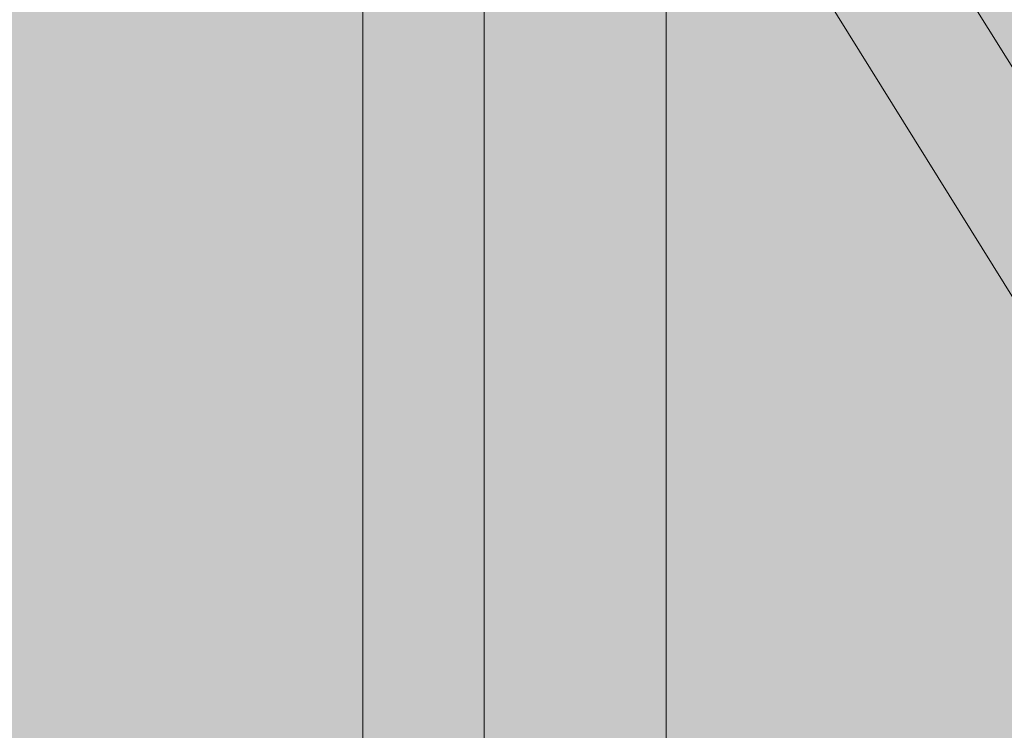
# Model space of a CAD drawing. Units: millimetres. Extents: x 11032 to 26788, y 3406 to 24505.
# Tile 45 of 78: x 15518 to 15924, y 15746 to 16039. Entities that reach past the tile are written whole.
import ezdxf

# ---------------------------------------------------------------- set-up
doc = ezdxf.new("R2010")
doc.units = ezdxf.units.MM
doc.header["$MEASUREMENT"] = 0
for name, color, linetype, lineweight in [('A-ANNO-DIMS', 2, 'Continuous', 18), ('A-GLAZ', 250, 'Continuous', 20), ('A-ROOF', 7, 'Continuous', 30), ('A-WALL', 7, 'Continuous', 35)]:
    doc.layers.add(name, color=color, linetype=linetype, lineweight=lineweight)
for name, color, linetype, lineweight, true_color in [('A-GLAZ-FRAM-PATT', 250, 'Continuous', 13, 0x262627), ('A-ROOF-PATT', 9, 'Continuous', 13, 0xc7c8ca), ('A-WALL-INTR-PATT', 251, 'Continuous', 13, 0x6c6b6a)]:
    doc.layers.add(name, color=color, linetype=linetype, lineweight=lineweight, true_color=true_color)
doc.styles.get("Standard").update_dxf_attribs({"font": 'arial.ttf'})
doc.dimstyles.get("Standard").update_dxf_attribs({"dimtxt": 150, "dimasz": 100, "dimexe": 10, "dimexo": 5, "dimgap": 5, "dimtad": 0, "dimtih": 1, "dimtoh": 1, "dimdec": 0, "dimzin": 0, "dimdsep": 46, "dimtxsty": 'Standard', "dimcen": 0.09, "dimadec": 0, "dimazin": 0, "dimtfac": 1, "dimtdec": 0, "dimtofl": 0, "dimtmove": 0, "dimatfit": 3, "dimfxl": 1, "dimtolj": 1, "dimtzin": 0, "dimarcsym": 0})

# ---------------------------------------------------------------- blocks, each defined once
blk = doc.blocks.new('*D36')
at = {"layer": 'A-ANNO-DIMS', "color": 0, "lineweight": -2, "transparency": 16777216}
for p, q in [((12301.26, 17115.89), (12301.26, 24416.86)), ((25397.4, 4466.4), (25397.4, 24416.86)), ((12401.26, 24406.86), (18569.2, 24406.86)), ((25297.4, 24406.86), (19129.47, 24406.86))]:
    blk.add_line(p, q, dxfattribs=at)
at = {"layer": 'A-ANNO-DIMS', "color": 0, "transparency": 16777216}
for points in [[(12401.26, 24423.52), (12401.26, 24390.19), (12301.26, 24406.86)], [(25297.4, 24423.52), (25297.4, 24390.19), (25397.4, 24406.86)]]:
    blk.add_solid(points, dxfattribs=at)
at = {"layer": 'Defpoints', "color": 0, "transparency": 16777216}
for p in [(25397.4, 24406.86), (12301.26, 17110.89), (25397.4, 4461.4)]:
    blk.add_point(p, dxfattribs=at)
at = {"layer": 'A-ANNO-DIMS', "color": 0, "transparency": 16777216, "insert": (18849.33, 24406.86), "char_height": 150, "attachment_point": 5}
blk.add_mtext('\\A1;13096', dxfattribs=at)
blk = doc.blocks.new('*D37')
at = {"layer": 'A-ANNO-DIMS', "color": 0, "lineweight": -2, "transparency": 16777216}
for p, q in [((18087.74, 23450.36), (11334.76, 23450.36)), ((11344.76, 23350.36), (11344.76, 14037.46)), ((11344.76, 4561.4), (11344.76, 13874.29)), ((12927.66, 4461.4), (11334.76, 4461.4))]:
    blk.add_line(p, q, dxfattribs=at)
at = {"layer": 'A-ANNO-DIMS', "color": 0, "transparency": 16777216}
for points in [[(11328.1, 23350.36), (11361.43, 23350.36), (11344.76, 23450.36)], [(11328.1, 4561.4), (11361.43, 4561.4), (11344.76, 4461.4)]]:
    blk.add_solid(points, dxfattribs=at)
at = {"layer": 'Defpoints', "color": 0, "transparency": 16777216}
for p in [(11344.76, 23450.36), (18092.74, 23450.36), (12932.66, 4461.4)]:
    blk.add_point(p, dxfattribs=at)
at = {"layer": 'A-ANNO-DIMS', "color": 0, "transparency": 16777216, "insert": (11344.76, 13955.88), "char_height": 150, "attachment_point": 5}
blk.add_mtext('\\A1;18989', dxfattribs=at)
blk = doc.blocks.new('*D57')
at = {"layer": 'A-ANNO-DIMS', "color": 0, "lineweight": -2, "transparency": 16777216}
for p, q in [((14994.7, 7266.4), (14994.7, 24416.86)), ((20894.7, 7266.4), (20894.7, 24416.86)), ((15094.7, 24406.86), (17715.98, 24406.86)), ((20794.7, 24406.86), (18173.42, 24406.86))]:
    blk.add_line(p, q, dxfattribs=at)
at = {"layer": 'A-ANNO-DIMS', "color": 0, "transparency": 16777216}
for points in [[(15094.7, 24423.52), (15094.7, 24390.19), (14994.7, 24406.86)], [(20794.7, 24423.52), (20794.7, 24390.19), (20894.7, 24406.86)]]:
    blk.add_solid(points, dxfattribs=at)
at = {"layer": 'Defpoints', "color": 0, "transparency": 16777216}
for p in [(20894.7, 24406.86), (14994.7, 7261.4), (20894.7, 7261.4)]:
    blk.add_point(p, dxfattribs=at)
at = {"layer": 'A-ANNO-DIMS', "color": 0, "transparency": 16777216, "insert": (17944.7, 24406.86), "char_height": 150, "attachment_point": 5}
blk.add_mtext('\\A1;5900', dxfattribs=at)
blk = doc.blocks.new('*D60')
at = {"layer": 'A-ANNO-DIMS', "color": 0, "lineweight": -2, "transparency": 16777216}
for p, q in [((14994.7, 7266.4), (14994.7, 24416.86)), ((16344.7, 7266.4), (16344.7, 24416.86)), ((15094.7, 24406.86), (15448.04, 24406.86)), ((16244.7, 24406.86), (15891.36, 24406.86))]:
    blk.add_line(p, q, dxfattribs=at)
at = {"layer": 'A-ANNO-DIMS', "color": 0, "transparency": 16777216}
for points in [[(15094.7, 24423.52), (15094.7, 24390.19), (14994.7, 24406.86)], [(16244.7, 24423.52), (16244.7, 24390.19), (16344.7, 24406.86)]]:
    blk.add_solid(points, dxfattribs=at)
at = {"layer": 'Defpoints', "color": 0, "transparency": 16777216}
for p in [(16344.7, 24406.86), (14994.7, 7261.4), (16344.7, 7261.4)]:
    blk.add_point(p, dxfattribs=at)
at = {"layer": 'A-ANNO-DIMS', "color": 0, "transparency": 16777216, "insert": (15669.7, 24406.86), "char_height": 150, "attachment_point": 5}
blk.add_mtext('\\A1;1350', dxfattribs=at)

msp = doc.modelspace()

# ---------------------------------------------------------------- hatches: boundary and pattern name
at = {"layer": 'A-GLAZ-FRAM-PATT'}
h = msp.add_hatch(color=256, dxfattribs=at)
edge = h.paths.add_edge_path()
edge.add_line((15284.393, 17051.32), (15084.393, 17001.32))
edge.add_line((15084.393, 17001.32), (15084.393, 15951.32))
edge.add_spline(control_points=[(15084.393, 15951.32), (15157.266, 15924.219), (15224.458, 15897.808), (15284.393, 15870.289)], knot_values=[511.9490104, 511.9490104, 511.9490104, 511.9490104, 697.3715979, 697.3715979, 697.3715979, 697.3715979], degree=3, periodic=0)
edge.add_line((15284.393, 15870.289), (15284.393, 17051.32))
edge = h.paths.add_edge_path()
edge.add_line((15659.393, 16354.387), (15459.393, 16675.629))
edge.add_line((15459.393, 16675.629), (15459.393, 15771.505))
edge.add_spline(control_points=[(15459.393, 15771.505), (15501.891, 15741.568), (15571.096, 15682.692), (15632.72, 15612.509), (15659.393, 15578.299)], knot_values=[905.064582, 905.064582, 905.064582, 905.064582, 1079.4682707, 1223.1584353, 1223.1584353, 1223.1584353, 1223.1584353], degree=3, periodic=0)
edge.add_line((15659.393, 15578.299), (15659.393, 16354.387))
h.paths.add_polyline_path([(15284.393, 17051.32), (15284.393, 16956.717), (15784.393, 16153.61), (15784.393, 16248.213)])
h = msp.add_hatch(color=256, dxfattribs=at)
edge = h.paths.add_edge_path()
edge.add_spline(control_points=[(15409.393, 16728.446), (15384.197, 16718.122), (15359.177, 16707.259), (15334.393, 16695.842)], knot_values=[2052.6714029, 2052.6714029, 2052.6714029, 2052.6714029, 2131.0201637, 2131.0201637, 2131.0201637, 2131.0201637], degree=3, periodic=0)
edge.add_line((15334.393, 16695.842), (15334.393, 15846.165))
edge.add_spline(control_points=[(15334.393, 15846.165), (15360.99, 15832.635), (15385.89, 15818.741), (15409.393, 15804.345)], knot_values=[750.8383504, 750.8383504, 750.8383504, 750.8383504, 839.4758736, 839.4758736, 839.4758736, 839.4758736], degree=3, periodic=0)
edge.add_line((15409.393, 15804.345), (15409.393, 16728.446))
edge = h.paths.add_edge_path()
edge.add_line((15784.393, 16153.61), (15709.393, 16274.076))
edge.add_line((15709.393, 16274.076), (15709.393, 15509.31))
edge.add_spline(control_points=[(15709.393, 15509.31), (15712.398, 15504.862), (15738.373, 15465.922), (15763.422, 15424.165), (15784.393, 15385.996)], knot_values=[1315.3424293, 1315.3424293, 1315.3424293, 1315.3424293, 1332.3824154, 1463.2850479, 1463.2850479, 1463.2850479, 1463.2850479], degree=3, periodic=0)
edge.add_line((15784.393, 15385.996), (15784.393, 16153.61))
h = msp.add_hatch(color=256, dxfattribs=at)
edge = h.paths.add_edge_path()
edge.add_line((15784.393, 16248.213), (15784.393, 16153.61))
edge.add_line((15784.393, 16153.61), (16560.042, 14907.752))
edge.add_spline(control_points=[(16560.042, 14907.752), (16569.192, 14907.664), (16578.343, 14907.575), (16587.493, 14907.486), (16598.103, 14907.383), (16608.713, 14907.281), (16619.296, 14907.181)], knot_values=[1012.2878735, 1012.2878735, 1012.2878735, 1012.2878735, 1027.155312, 1027.155312, 1027.155312, 1044.3939449, 1044.3939449, 1044.3939449, 1044.3939449], degree=3, periodic=0)
edge.add_line((16619.296, 14907.181), (15784.393, 16248.213))
at = {"layer": 'A-ROOF-PATT'}
h = msp.add_hatch(color=256, dxfattribs=at)
edge = h.paths.add_edge_path()
edge.add_spline(control_points=[(17532.827, 17324.837), (17391.335, 17349.016), (16840.872, 17494.912), (16080.055, 18069.544), (14738.803, 18299.641), (13382.429, 18838.336), (12580.532, 17870.207), (12430.422, 17563.822)], knot_values=[2977.6027945, 2977.6027945, 2977.6027945, 2977.6027945, 3438.1840601, 4811.6463022, 5622.8675483, 7588.0288188, 8560.6685791, 8560.6685791, 8560.6685791, 8560.6685791], degree=3, periodic=0)
edge.add_spline(control_points=[(12430.422, 17563.822), (12437.904, 17573.36), (12445.386, 17582.899), (12452.869, 17592.437), (12452.869, 17592.438), (12452.869, 17592.438), (12452.869, 17592.438)], knot_values=[1408.564138, 1408.564138, 1408.564138, 1408.564138, 1444.85989, 1444.85989, 1444.85989, 1444.8601183, 1444.8601183, 1444.8601183, 1444.8601183], degree=3, periodic=0)
edge.add_spline(control_points=[(12452.869, 17592.438), (12555.432, 17723.185), (12736.557, 17929.686), (13044.86, 18114.643), (13219.943, 18189.644), (13299.92, 18220.646)], knot_values=[339.318246, 339.318246, 339.318246, 339.318246, 836.8349967, 1151.2512933, 1408.564138, 1408.564138, 1408.564138, 1408.564138], degree=3, periodic=0)
edge.add_spline(control_points=[(13299.92, 18220.646), (13299.998, 18220.689), (13300.077, 18220.732), (13319.738, 18231.488), (13339.24, 18241.402), (13388.645, 18264.703), (13418.466, 18277.069), (13478.019, 18298.648), (13507.751, 18307.861), (13544.561, 18317.488), (13551.584, 18319.245), (13558.612, 18320.924)], knot_values=[3783.8950972, 3783.8950972, 3783.8950972, 3783.8950972, 3784.1737101, 3784.1737101, 3853.4666747, 3853.4666747, 3960.2401917, 3960.2401917, 4067.0137087, 4067.0137087, 4092.1744649, 4092.1744649, 4092.1744649, 4092.1744649], degree=3, periodic=0)
edge.add_spline(control_points=[(13558.612, 18320.924), (13581.407, 18326.373), (13604.25, 18331.007), (13657.184, 18339.957), (13687.338, 18343.732), (13748.098, 18348.892), (13778.704, 18350.276), (13840.46, 18350.833), (13871.609, 18350.005), (13934.496, 18346.313), (13966.232, 18343.449), (14030.297, 18335.871), (14062.625, 18331.158), (14127.853, 18320.088), (14160.753, 18313.73), (14241.357, 18296.556), (14289.343, 18284.997), (14386.31, 18259.688), (14435.291, 18245.941), (14534.161, 18217.034), (14584.049, 18201.875), (14684.682, 18170.964), (14735.427, 18155.212), (14837.763, 18123.971), (14889.354, 18108.482), (14954.971, 18089.677), (14968.586, 18085.823), (14992.391, 18079.184), (15002.566, 18076.376), (15021.739, 18071.153), (15030.731, 18068.729), (15047.707, 18064.21), (15055.694, 18062.106), (15079.815, 18055.825), (15095.905, 18051.728), (15143.966, 18039.717), (15175.729, 18032.084), (15254.84, 18013.501), (15301.798, 18002.866), (15394.186, 17981.845), (15439.615, 17971.459), (15528.833, 17950.135), (15572.62, 17939.197), (15658.477, 17916.021), (15700.546, 17903.785), (15753.633, 17886.734), (15765.446, 17882.835), (15786.574, 17875.653), (15795.915, 17872.404), (15810.108, 17867.349), (15814.99, 17865.588), (15824.736, 17862.029), (15829.611, 17860.226), (15844.241, 17854.75), (15854.002, 17851.008), (15883.312, 17839.521), (15902.885, 17831.512), (15966.355, 17804.548), (16010.39, 17784.302), (16098.838, 17741.267), (16143.25, 17718.478), (16232.497, 17671.098), (16277.332, 17646.507), (16367.515, 17596.295), (16412.862, 17570.676), (16504.202, 17519.209), (16550.194, 17493.362), (16643.009, 17442.263), (16689.831, 17417.011), (16756.517, 17382.472), (16775.937, 17372.58), (16795.455, 17362.84)], knot_values=[4092.1744649, 4092.1744649, 4092.1744649, 4092.1744649, 4173.7872258, 4173.7872258, 4280.5607428, 4280.5607428, 4387.3342598, 4387.3342598, 4494.1077768, 4494.1077768, 4600.8812939, 4600.8812939, 4707.6548109, 4707.6548109, 4814.4283279, 4814.4283279, 4967.1262405, 4967.1262405, 5119.8241531, 5119.8241531, 5272.5220657, 5272.5220657, 5425.2199783, 5425.2199783, 5577.9178908, 5577.9178908, 5617.7853319, 5617.7853319, 5647.4648479, 5647.4648479, 5673.611025, 5673.611025, 5696.747607, 5696.747607, 5743.6818903, 5743.6818903, 5837.5504571, 5837.5504571, 5979.7261046, 5979.7261046, 6121.9017521, 6121.9017521, 6264.0773996, 6264.0773996, 6406.2530471, 6406.2530471, 6447.2585849, 6447.2585849, 6480.0420882, 6480.0420882, 6497.3077062, 6497.3077062, 6514.5733242, 6514.5733242, 6549.1045602, 6549.1045602, 6618.1670322, 6618.1670322, 6772.6610171, 6772.6610171, 6927.155002, 6927.155002, 7081.6489869, 7081.6489869, 7236.1429718, 7236.1429718, 7390.6369567, 7390.6369567, 7545.1309416, 7545.1309416, 7608.1992868, 7608.1992868, 7608.1992868, 7608.1992868], degree=3, periodic=0)
edge.add_spline(control_points=[(16795.455, 17362.84), (16814.335, 17349.456), (16832.897, 17336.263), (16873.225, 17307.197), (16894.778, 17291.386), (16936.221, 17259.941), (16956.11, 17244.308), (16993.863, 17213.094), (17011.726, 17197.514), (17041.993, 17169.265), (17054.791, 17156.601), (17078.762, 17131.225), (17089.933, 17118.516), (17110.618, 17092.991), (17120.131, 17080.178), (17130.17, 17065.264), (17131.487, 17063.277), (17133.77, 17059.776), (17134.746, 17058.261), (17136.69, 17055.205), (17137.657, 17053.668), (17140.539, 17049.025), (17142.438, 17045.89), (17148.068, 17036.367), (17151.732, 17029.859), (17163.03, 17008.788), (17170.335, 16993.646), (17184.087, 16961.978), (17190.534, 16945.453), (17202.562, 16911.165), (17208.142, 16893.402), (17218.448, 16856.821), (17223.173, 16838.003), (17231.801, 16799.51), (17235.705, 16779.837), (17241.533, 16746.739), (17243.676, 16733.5), (17247.718, 16706.37), (17249.608, 16692.472), (17252.066, 16672.69), (17252.761, 16666.875), (17254.1, 16655.226), (17254.744, 16649.4), (17256.596, 16631.917), (17257.727, 16620.254), (17260.823, 16585.238), (17262.489, 16561.858), (17266.551, 16488.654), (17267.658, 16438.661), (17267.349, 16375.228), (17267.193, 16362.07), (17266.95, 16348.891)], knot_values=[15.1130472, 15.1130472, 15.1130472, 15.1130472, 82.6995146, 82.6995146, 165.3990291, 165.3990291, 248.0985437, 248.0985437, 330.7980583, 330.7980583, 397.9419458, 397.9419458, 465.0858333, 465.0858333, 532.2297209, 532.2297209, 542.533741, 542.533741, 550.3568158, 550.3568158, 558.1798906, 558.1798906, 573.8260402, 573.8260402, 605.1183395, 605.1183395, 672.7640614, 672.7640614, 740.4097834, 740.4097834, 808.0555054, 808.0555054, 875.7012273, 875.7012273, 943.3469493, 943.3469493, 987.6613492, 987.6613492, 1033.4121612, 1033.4121612, 1052.3850876, 1052.3850876, 1071.358014, 1071.358014, 1109.3038668, 1109.3038668, 1185.1955724, 1185.1955724, 1346.4419026, 1346.4419026, 1388.5586631, 1388.5586631, 1388.5586631, 1388.5586631], degree=3, periodic=0)
edge.add_spline(control_points=[(17266.95, 16348.891), (17266.95, 16348.891), (17266.95, 16348.891), (17266.95, 16348.891), (17253.182, 15602.417), (17239.414, 14855.943), (17225.646, 14109.469)], knot_values=[1388.5586631, 1388.5586631, 1388.5586631, 1388.5586631, 1388.5589654, 1388.5589654, 1388.5589654, 3774.0767661, 3774.0767661, 3774.0767661, 3774.0767661], degree=3, periodic=0)
edge.add_spline(control_points=[(17225.646, 14109.469), (17226.198, 14109.827), (17226.748, 14110.185), (17242.065, 14120.191), (17255.956, 14130.116), (17274.422, 14144.286), (17279.609, 14148.386), (17284.686, 14152.511)], knot_values=[1926.3423968, 1926.3423968, 1926.3423968, 1926.3423968, 1927.316729, 1927.316729, 1953.5121761, 1953.5121761, 1964.0732348, 1964.0732348, 1964.0732348, 1964.0732348], degree=3, periodic=0)
edge.add_spline(control_points=[(17284.686, 14152.511), (17315.791, 14194.761), (17384.413, 14446.273), (17407.128, 14793.401), (17407.093, 15295.84), (17423.274, 15626.362), (17415.601, 15782.507)], knot_values=[0, 0, 0, 0, 163.2554674, 619.2296767, 1171.8624483, 1621.6355562, 1621.6355562, 1621.6355562, 1621.6355562], degree=3, periodic=0)
edge.add_spline(control_points=[(17415.601, 15782.507), (17438.21, 16077.57), (17410.495, 16533.484), (17390.893, 17030.649), (17301.082, 17169.349)], knot_values=[543.9784753, 543.9784753, 543.9784753, 543.9784753, 1452.9852767, 1960.0114926, 1960.0114926, 1960.0114926, 1960.0114926], degree=3, periodic=0)
edge.add_spline(control_points=[(17301.082, 17169.349), (17346.58, 17157.64), (17392.235, 17147.336), (17467.161, 17132.609), (17496.336, 17127.412), (17525.58, 17122.709)], knot_values=[8131.593939, 8131.593939, 8131.593939, 8131.593939, 8269.7349273, 8269.7349273, 8357.5016646, 8357.5016646, 8357.5016646, 8357.5016646], degree=3, periodic=0)
edge.add_line((17525.58, 17122.709), (17532.827, 17324.837))
edge = h.paths.add_edge_path(flags=17)
edge.add_spline(control_points=[(13340.537, 14602.706), (13316.172, 14726.456), (13323.666, 14932.342), (13637.836, 15081.117), (13863.248, 15171.051), (14002.1, 15224.503), (14058.539, 15244.876)], knot_values=[680.8931862, 680.8931862, 680.8931862, 680.8931862, 1033.4728289, 1337.4008326, 1604.7214264, 1784.2944722, 1784.2944722, 1784.2944722, 1784.2944722], degree=3, periodic=0)
edge.add_spline(control_points=[(14058.539, 15244.876), (14058.289, 15275.236), (14057.634, 15305.434), (14055.312, 15376.527), (14053.359, 15417.248), (14048.642, 15497.048), (14045.89, 15536.143), (14042.888, 15574.619)], knot_values=[6573.1065419, 6573.1065419, 6573.1065419, 6573.1065419, 6636.7330012, 6636.7330012, 6723.8890547, 6723.8890547, 6809.6328771, 6809.6328771, 6809.6328771, 6809.6328771], degree=3, periodic=0)
edge.add_spline(control_points=[(14042.888, 15574.619), (13546.54, 15403.221), (13074.735, 15143.241), (13277.36, 14695.339), (13340.537, 14602.706)], knot_values=[503.7925783, 503.7925783, 503.7925783, 503.7925783, 1728.1787606, 2051.34844, 2051.34844, 2051.34844, 2051.34844], degree=3, periodic=0)
h = msp.add_hatch(color=256, dxfattribs=at)
h.set_gradient(color1=(254, 234, 185), color2=(254, 204, 102), name='HEMISPHERICAL')
edge = h.paths.add_edge_path()
edge.add_line((15084.393, 17001.32), (15284.393, 17051.32))
edge.add_line((15284.393, 17051.32), (15470.537, 16752.334))
edge.add_spline(control_points=[(15470.537, 16752.334), (15683.311, 16831.508), (16106.827, 16912.335), (16625.609, 16876.997), (17083.498, 16357.78), (17257.801, 16180.113)], knot_values=[0, 0, 0, 0, 655.2936334, 1252.0157838, 1989.6162859, 1989.6162859, 1989.6162859, 1989.6162859], degree=3, periodic=0)
edge.add_spline(control_points=[(17257.801, 16180.113), (17260.851, 16236.372), (17263.9, 16292.632), (17266.95, 16348.891)], knot_values=[1132.9967717, 1132.9967717, 1132.9967717, 1132.9967717, 1198.0464225, 1198.0464225, 1198.0464225, 1198.0464225], degree=3, periodic=0)
edge.add_spline(control_points=[(17266.95, 16348.891), (17267.193, 16362.07), (17267.349, 16375.228), (17267.658, 16438.661), (17266.551, 16488.654), (17262.489, 16561.858), (17260.823, 16585.238), (17257.727, 16620.254), (17256.596, 16631.917), (17254.744, 16649.4), (17254.1, 16655.226), (17252.761, 16666.875), (17252.066, 16672.69), (17249.608, 16692.472), (17247.718, 16706.37), (17243.676, 16733.5), (17241.533, 16746.739), (17235.705, 16779.837), (17231.801, 16799.51), (17223.173, 16838.003), (17218.448, 16856.821), (17208.142, 16893.402), (17202.562, 16911.165), (17190.534, 16945.453), (17184.087, 16961.978), (17170.335, 16993.646), (17163.03, 17008.788), (17151.732, 17029.859), (17148.068, 17036.367), (17142.438, 17045.89), (17140.539, 17049.025), (17137.657, 17053.668), (17136.69, 17055.205), (17134.746, 17058.261), (17133.77, 17059.776), (17131.487, 17063.277), (17130.17, 17065.264), (17120.131, 17080.178), (17110.618, 17092.991), (17089.933, 17118.516), (17078.762, 17131.225), (17054.791, 17156.601), (17041.993, 17169.265), (17011.726, 17197.514), (16993.863, 17213.094), (16956.11, 17244.308), (16936.221, 17259.941), (16894.778, 17291.386), (16873.225, 17307.197), (16832.897, 17336.263), (16814.335, 17349.456), (16795.455, 17362.84)], knot_values=[15.1130472, 15.1130472, 15.1130472, 15.1130472, 57.2298077, 57.2298077, 218.4761379, 218.4761379, 294.3678435, 294.3678435, 332.3136963, 332.3136963, 351.2866227, 351.2866227, 370.2595491, 370.2595491, 416.0103612, 416.0103612, 460.324761, 460.324761, 527.970483, 527.970483, 595.616205, 595.616205, 663.2619269, 663.2619269, 730.9076489, 730.9076489, 798.5533709, 798.5533709, 829.8456701, 829.8456701, 845.4918197, 845.4918197, 853.3148945, 853.3148945, 861.1379693, 861.1379693, 871.4419895, 871.4419895, 938.585877, 938.585877, 1005.7297645, 1005.7297645, 1072.8736521, 1072.8736521, 1155.5731666, 1155.5731666, 1238.2726812, 1238.2726812, 1320.9721958, 1320.9721958, 1388.5586631, 1388.5586631, 1388.5586631, 1388.5586631], degree=3, periodic=0)
edge.add_spline(control_points=[(16795.455, 17362.84), (16775.937, 17372.58), (16756.517, 17382.472), (16689.831, 17417.011), (16643.009, 17442.263), (16550.194, 17493.362), (16504.202, 17519.209), (16412.862, 17570.676), (16367.515, 17596.295), (16277.332, 17646.507), (16232.497, 17671.098), (16143.25, 17718.478), (16098.838, 17741.267), (16010.39, 17784.302), (15966.355, 17804.548), (15902.885, 17831.512), (15883.312, 17839.521), (15854.002, 17851.008), (15844.241, 17854.75), (15829.611, 17860.226), (15824.736, 17862.029), (15814.99, 17865.588), (15810.108, 17867.349), (15795.915, 17872.404), (15786.574, 17875.653), (15765.446, 17882.835), (15753.633, 17886.734), (15700.546, 17903.785), (15658.477, 17916.021), (15572.62, 17939.197), (15528.833, 17950.135), (15439.615, 17971.459), (15394.186, 17981.845), (15301.798, 18002.866), (15254.84, 18013.501), (15175.729, 18032.084), (15143.966, 18039.717), (15095.905, 18051.728), (15079.815, 18055.825), (15055.694, 18062.106), (15047.707, 18064.21), (15030.731, 18068.729), (15021.739, 18071.153), (15002.566, 18076.376), (14992.391, 18079.184), (14968.586, 18085.823), (14954.971, 18089.677), (14889.354, 18108.482), (14837.763, 18123.971), (14735.427, 18155.212), (14684.682, 18170.964), (14584.049, 18201.875), (14534.161, 18217.034), (14435.291, 18245.941), (14386.31, 18259.688), (14289.343, 18284.997), (14241.357, 18296.556), (14160.753, 18313.73), (14127.853, 18320.088), (14062.625, 18331.158), (14030.297, 18335.871), (13966.232, 18343.449), (13934.496, 18346.313), (13871.609, 18350.005), (13840.46, 18350.833), (13778.704, 18350.276), (13748.098, 18348.892), (13687.338, 18343.732), (13657.184, 18339.957), (13604.25, 18331.007), (13581.407, 18326.373), (13558.612, 18320.924)], knot_values=[4092.1744649, 4092.1744649, 4092.1744649, 4092.1744649, 4155.2428101, 4155.2428101, 4309.736795, 4309.736795, 4464.2307799, 4464.2307799, 4618.7247648, 4618.7247648, 4773.2187497, 4773.2187497, 4927.7127346, 4927.7127346, 5082.2067195, 5082.2067195, 5151.2691915, 5151.2691915, 5185.8004275, 5185.8004275, 5203.0660455, 5203.0660455, 5220.3316635, 5220.3316635, 5253.1151668, 5253.1151668, 5294.1207046, 5294.1207046, 5436.2963521, 5436.2963521, 5578.4719996, 5578.4719996, 5720.6476471, 5720.6476471, 5862.8232946, 5862.8232946, 5956.6918614, 5956.6918614, 6003.6261447, 6003.6261447, 6026.7627267, 6026.7627267, 6052.9089038, 6052.9089038, 6082.5884198, 6082.5884198, 6122.4558609, 6122.4558609, 6275.1537734, 6275.1537734, 6427.851686, 6427.851686, 6580.5495986, 6580.5495986, 6733.2475112, 6733.2475112, 6885.9454238, 6885.9454238, 6992.7189408, 6992.7189408, 7099.4924578, 7099.4924578, 7206.2659749, 7206.2659749, 7313.0394919, 7313.0394919, 7419.8130089, 7419.8130089, 7526.5865259, 7526.5865259, 7608.1992868, 7608.1992868, 7608.1992868, 7608.1992868], degree=3, periodic=0)
edge.add_spline(control_points=[(13558.612, 18320.924), (13472.381, 18287.498), (13386.15, 18254.072), (13299.92, 18220.646), (13299.92, 18220.646), (13299.92, 18220.646), (13299.92, 18220.646)], knot_values=[61.8832457, 61.8832457, 61.8832457, 61.8832457, 339.3179746, 339.3179746, 339.3179746, 339.318246, 339.318246, 339.318246, 339.318246], degree=3, periodic=0)
edge.add_spline(control_points=[(13299.92, 18220.646), (13219.943, 18189.644), (13044.86, 18114.643), (12736.557, 17929.686), (12555.432, 17723.185), (12452.869, 17592.438)], knot_values=[339.318246, 339.318246, 339.318246, 339.318246, 596.6310906, 911.0473872, 1408.564138, 1408.564138, 1408.564138, 1408.564138], degree=3, periodic=0)
edge.add_spline(control_points=[(12452.869, 17592.438), (12452.869, 17592.438), (12452.869, 17592.438), (12452.869, 17592.437), (12445.386, 17582.899), (12437.904, 17573.36), (12430.422, 17563.822)], knot_values=[1408.564138, 1408.564138, 1408.564138, 1408.564138, 1408.5643663, 1408.5643663, 1408.5643663, 1444.8601183, 1444.8601183, 1444.8601183, 1444.8601183], degree=3, periodic=0)
edge.add_spline(control_points=[(12430.422, 17563.822), (12373.797, 17448.248), (12157.302, 16836.764), (12751.985, 16393.69), (13424.325, 15907.903), (14042.888, 15574.619)], knot_values=[0, 0, 0, 0, 366.8993034, 1975.5941082, 2977.6027945, 2977.6027945, 2977.6027945, 2977.6027945], degree=3, periodic=0)
edge.add_spline(control_points=[(14042.888, 15574.619), (14042.839, 15575.252), (14042.789, 15575.886), (14039.681, 15615.607), (14036.366, 15654.052), (14029.551, 15729.305), (14026.05, 15766.114), (14019.175, 15837.686), (14015.8, 15872.45), (13903.823, 16338.596)], knot_values=[6310.2261504, 6310.2261504, 6310.2261504, 6310.2261504, 6311.6383814, 6311.6383814, 6398.7944349, 6398.7944349, 6485.9504884, 6485.9504884, 6573.1065419, 6573.1065419, 6573.1065419, 6573.1065419], degree=3, periodic=0)
edge.add_spline(control_points=[(13903.823, 16338.596), (14237.315, 16236.889), (14456.623, 16167.555), (14614.196, 16115.84)], knot_values=[0, 0, 0, 0, 202.9853419, 202.9853419, 202.9853419, 202.9853419], degree=3, periodic=0)
edge.add_spline(control_points=[(14614.196, 16115.84), (14663.209, 16178.992), (14799.965, 16341.237), (14969.915, 16481.426), (15084.393, 16556.825)], knot_values=[2405.0345045, 2405.0345045, 2405.0345045, 2405.0345045, 2644.8826966, 3039.2707272, 3039.2707272, 3039.2707272, 3039.2707272], degree=3, periodic=0)
edge.add_line((15084.393, 16556.825), (15084.393, 17001.32))
h.paths.add_polyline_path([(14195.599, 17606.181, -1), (14395.599, 17606.181, -1)], flags=16)
h.paths.add_polyline_path([(13310.178, 17032.97, -1), (13510.178, 17032.97, -1)], flags=16)
h = msp.add_hatch(color=256, dxfattribs=at)
h.set_gradient(color1=(254, 234, 185), color2=(254, 204, 102), name='HEMISPHERICAL')
edge = h.paths.add_edge_path()
edge.add_spline(control_points=[(16560.042, 14907.752), (16569.192, 14907.664), (16578.343, 14907.575), (16587.493, 14907.486), (16832.101, 14905.115), (17122.895, 14902.296), (16849.359, 14976.117), (16870.954, 15304.114), (17098.337, 15241.178), (17235.385, 15203.245)], knot_values=[0, 0, 0, 0, 14.8674385, 14.8674385, 14.8674385, 412.2943091, 487.3345915, 708.6416004, 1044.3939449, 1044.3939449, 1044.3939449, 1044.3939449], degree=3, periodic=0)
edge.add_line((16587.504, 14907.486), (16560.207, 14907.486))
edge.add_line((16560.207, 14907.486), (15784.393, 16153.61))
edge.add_line((15784.393, 16153.61), (15784.393, 15385.996))
edge.add_spline(control_points=[(15784.393, 15385.996), (15798.391, 15360.52), (15847.198, 15266.214), (15887.196, 15168.614), (15912.903, 15096.727)], knot_values=[1463.2850479, 1463.2850479, 1463.2850479, 1463.2850479, 1550.659771, 1779.9599361, 1779.9599361, 1779.9599361, 1779.9599361], degree=3, periodic=0)
edge.add_spline(control_points=[(15912.903, 15096.727), (15913.652, 15095.649), (15914.403, 15094.565), (15925.191, 15078.948), (15935.516, 15063.47), (15956.582, 15030.918), (15967.324, 15013.844), (15989.119, 14978.386), (16000.173, 14960.003), (16022.525, 14922.193), (16033.824, 14902.767), (16056.63, 14863.116), (16068.138, 14842.891), (16091.349, 14801.871), (16103.053, 14781.075), (16126.666, 14739.118), (16138.575, 14717.958), (16162.628, 14675.459), (16174.772, 14654.12), (16199.352, 14611.428), (16211.787, 14590.075), (16237.037, 14547.491), (16249.851, 14526.26), (16271.946, 14490.566), (16281.092, 14476.044), (16299.694, 14447.129), (16309.149, 14432.737), (16328.456, 14404.098), (16338.307, 14389.85), (16358.518, 14361.503), (16368.879, 14347.403), (16390.266, 14319.347), (16401.291, 14305.391), (16420.626, 14281.969), (16428.703, 14272.467), (16445.363, 14253.527), (16453.946, 14244.088), (16471.727, 14225.278), (16480.926, 14215.907), (16500.075, 14197.247), (16510.026, 14187.959), (16530.844, 14169.504), (16541.71, 14160.337), (16564.549, 14142.195), (16576.522, 14133.22), (16597.69, 14118.448), (16606.528, 14112.565), (16624.87, 14101.004), (16634.376, 14095.326), (16654.117, 14084.255), (16664.352, 14078.862), (16685.603, 14068.46), (16696.619, 14063.452), (16719.46, 14053.944), (16731.285, 14049.444), (16755.742, 14041.097), (16768.374, 14037.251), (16794.396, 14030.368), (16807.787, 14027.332), (16835.229, 14022.23), (16849.279, 14020.163), (16877.882, 14017.141), (16892.435, 14016.186), (16921.835, 14015.489), (16936.683, 14015.749), (16961.564, 14017.241), (16971.582, 14018.127), (16986.57, 14019.883), (16991.56, 14020.54), (16999.027, 14021.63), (17001.514, 14022.011), (17006.48, 14022.809), (17008.962, 14023.225), (17014.824, 14024.251), (17018.193, 14024.875), (17036.262, 14028.398), (17050.55, 14031.826), (17078.171, 14039.583), (17091.505, 14043.912), (17115.643, 14052.705), (17126.557, 14057.089), (17137.108, 14061.688)], knot_values=[2010.7639617, 2010.7639617, 2010.7639617, 2010.7639617, 2014.7029827, 2014.7029827, 2067.238337, 2067.238337, 2119.7736913, 2119.7736913, 2172.3090457, 2172.3090457, 2224.8444, 2224.8444, 2277.3797543, 2277.3797543, 2329.9151086, 2329.9151086, 2382.450463, 2382.450463, 2434.9858173, 2434.9858173, 2487.5211716, 2487.5211716, 2540.0565259, 2540.0565259, 2576.3179289, 2576.3179289, 2612.5793318, 2612.5793318, 2648.8407347, 2648.8407347, 2685.1021376, 2685.1021376, 2721.3635405, 2721.3635405, 2746.252015, 2746.252015, 2771.1404895, 2771.1404895, 2796.028964, 2796.028964, 2820.9174385, 2820.9174385, 2845.8059131, 2845.8059131, 2870.6943876, 2870.6943876, 2887.5132757, 2887.5132757, 2904.3321639, 2904.3321639, 2921.1510521, 2921.1510521, 2937.9699402, 2937.9699402, 2954.7888284, 2954.7888284, 2971.6077166, 2971.6077166, 2988.4266047, 2988.4266047, 3005.2454929, 3005.2454929, 3022.0643811, 3022.0643811, 3038.8832692, 3038.8832692, 3050.1975453, 3050.1975453, 3055.8546833, 3055.8546833, 3058.6832524, 3058.6832524, 3061.5118214, 3061.5118214, 3065.3934173, 3065.3934173, 3082.4668716, 3082.4668716, 3099.5403259, 3099.5403259, 3114.5433443, 3114.5433443, 3114.5433443, 3114.5433443], degree=3, periodic=0)
edge.add_spline(control_points=[(17137.108, 14061.688), (17165.253, 14274.398), (17209.97, 14653.885), (17230.2, 15035.586), (17235.385, 15203.245)], knot_values=[1968.0804557, 1968.0804557, 1968.0804557, 1968.0804557, 2611.5282875, 3114.5379264, 3114.5379264, 3114.5379264, 3114.5379264], degree=3, periodic=0)
edge = h.paths.add_edge_path()
edge.add_spline(control_points=[(16856.103, 14956.992), (16852.841, 14961.219), (16849.83, 14965.576), (16842.539, 14977.287), (16838.658, 14984.798), (16832.033, 15000.109), (16829.289, 15007.911), (16824.126, 15026.008), (16822.047, 15036.354), (16819.308, 15057.097), (16818.649, 15067.496), (16818.576, 15088.188), (16819.162, 15098.483), (16821.467, 15118.823), (16823.186, 15128.868), (16827.696, 15148.567), (16830.486, 15158.22), (16836.065, 15173.969), (16838.565, 15180.211), (16844.079, 15192.402), (16847.092, 15198.353), (16852.029, 15207.021), (16853.744, 15209.868), (16857.321, 15215.468), (16859.188, 15218.226), (16863.017, 15223.558), (16864.978, 15226.136), (16872.565, 15235.558), (16878.593, 15241.952), (16891.428, 15253.591), (16898.232, 15258.834), (16912.397, 15268.127), (16919.756, 15272.176), (16934.816, 15279.138), (16942.515, 15282.052), (16958.1, 15286.873), (16965.985, 15288.78), (16984.013, 15292.142), (16994.186, 15293.334), (17014.631, 15294.619), (17024.904, 15294.713), (17048.453, 15293.935), (17061.76, 15292.783), (17088.519, 15289.422), (17101.972, 15287.211), (17131.961, 15281.46), (17148.526, 15277.734), (17181.692, 15269.627), (17198.292, 15265.245), (17222.182, 15258.759), (17229.535, 15256.737), (17236.862, 15254.714)], knot_values=[9.6639535, 9.6639535, 9.6639535, 9.6639535, 20.0351668, 20.0351668, 36.9411752, 36.9411752, 53.8471837, 53.8471837, 75.7795687, 75.7795687, 97.7119538, 97.7119538, 119.6443388, 119.6443388, 141.5767238, 141.5767238, 163.5091089, 163.5091089, 178.3829945, 178.3829945, 193.2568801, 193.2568801, 200.6938229, 200.6938229, 208.1307657, 208.1307657, 215.4448585, 215.4448585, 235.5795923, 235.5795923, 255.7143261, 255.7143261, 275.8490598, 275.8490598, 295.9837936, 295.9837936, 316.1185274, 316.1185274, 341.7220543, 341.7220543, 367.3255812, 367.3255812, 400.1572431, 400.1572431, 432.988905, 432.988905, 473.0440165, 473.0440165, 513.099128, 513.099128, 530.9692999, 530.9692999, 530.9692999, 530.9692999], degree=3, periodic=0)
edge.add_spline(control_points=[(17236.862, 15254.714), (17240.377, 15387.456), (17242.496, 15609.536), (17239.752, 15831.567), (17250.544, 16044.717)], knot_values=[1250.9818616, 1250.9818616, 1250.9818616, 1250.9818616, 1649.1516581, 1916.613987, 1916.613987, 1916.613987, 1916.613987], degree=3, periodic=0)
edge.add_spline(control_points=[(17250.544, 16044.717), (17229.169, 16066.505), (17207.794, 16088.292), (17186.419, 16110.08), (17186.418, 16110.08), (17186.418, 16110.081), (17186.418, 16110.081)], knot_values=[-88.5185581, -88.5185581, -88.5185581, -88.5185581, -0.0012784, -0.0012784, -0.0012784, 0, 0, 0, 0], degree=3, periodic=0)
edge.add_spline(control_points=[(17186.418, 16110.081), (17169.261, 16127.569), (17151.499, 16145.947), (17114.892, 16184.084), (17096.046, 16203.842), (17057.437, 16244.305), (17037.673, 16265.01), (16997.415, 16306.918), (16976.921, 16328.12), (16927.79, 16378.347), (16898.924, 16407.388), (16840.771, 16464.327), (16811.484, 16492.225), (16758.449, 16540.764), (16734.666, 16561.798), (16687.634, 16601.588), (16664.382, 16620.344), (16624.116, 16650.909), (16606.897, 16663.324), (16583.769, 16678.999), (16577.49, 16683.149), (16567.144, 16689.805), (16563.039, 16692.397), (16550.823, 16699.959), (16542.775, 16704.739), (16526.841, 16713.814), (16518.956, 16718.108), (16495.524, 16730.301), (16480.199, 16737.514), (16449.97, 16750.334), (16435.066, 16755.942), (16405.476, 16765.764), (16390.79, 16769.979), (16361.418, 16777.195), (16346.731, 16780.197), (16317.147, 16785.133), (16302.249, 16787.067), (16272.053, 16789.992), (16256.756, 16790.981), (16225.609, 16792.125), (16209.759, 16792.279), (16177.385, 16791.865), (16160.862, 16791.296), (16136.98, 16790.07), (16129.942, 16789.661), (16118.22, 16788.91), (16113.574, 16788.594), (16103.645, 16787.886), (16098.362, 16787.489), (16087.761, 16786.652), (16082.439, 16786.212), (16066.413, 16784.825), (16055.649, 16783.812), (16023.135, 16780.505), (16001.164, 16777.942), (15934.539, 16769.141), (15889.17, 16761.791), (15797.417, 16743.949), (15751.033, 16733.457), (15645.217, 16705.796), (15585.74, 16687.58), (15526.207, 16666.217), (15525.367, 16665.915), (15524.528, 16665.613)], knot_values=[0, 0, 0, 0, 71.0501454, 71.0501454, 142.1002909, 142.1002909, 213.1504363, 213.1504363, 284.2005818, 284.2005818, 381.323193, 381.323193, 478.4458043, 478.4458043, 557.8219847, 557.8219847, 637.1981651, 637.1981651, 698.3122593, 698.3122593, 721.3971375, 721.3971375, 736.7790891, 736.7790891, 767.5429924, 767.5429924, 798.3068957, 798.3068957, 859.8347022, 859.8347022, 921.3625088, 921.3625088, 982.8903154, 982.8903154, 1044.4181219, 1044.4181219, 1105.9459285, 1105.9459285, 1167.4737351, 1167.4737351, 1229.0015416, 1229.0015416, 1290.5293482, 1290.5293482, 1315.8990035, 1315.8990035, 1332.3812792, 1332.3812792, 1350.9052657, 1350.9052657, 1369.4292522, 1369.4292522, 1406.4772252, 1406.4772252, 1480.5731712, 1480.5731712, 1628.7650633, 1628.7650633, 1776.9569554, 1776.9569554, 1966.3109251, 1966.3109251, 1969.019495, 1969.019495, 1969.019495, 1969.019495], degree=3, periodic=0)
edge.add_line((15524.528, 16665.613), (16587.978, 14957.484))
edge.add_spline(control_points=[(16587.978, 14957.484), (16605.253, 14957.316), (16622.516, 14957.149), (16665.945, 14956.759), (16691.933, 14956.554), (16742.419, 14956.302), (16766.918, 14956.255), (16813.531, 14956.412), (16835.647, 14956.617), (16856.103, 14956.992)], knot_values=[872.2181925, 872.2181925, 872.2181925, 872.2181925, 900.2857301, 900.2857301, 943.3659889, 943.3659889, 986.4462476, 986.4462476, 1029.5265064, 1029.5265064, 1029.5265064, 1029.5265064], degree=3, periodic=0)
h.paths.add_polyline_path([(16474.605, 15622.642, -1), (16624.605, 15622.642, -1)], flags=16)
h.paths.add_polyline_path([(16198.536, 16037.613, -1), (16348.536, 16037.613, -1)], flags=16)
h.paths.add_polyline_path([(16475.717, 16408.125, -1), (16625.717, 16408.125, -1)], flags=16)
at = {"layer": 'A-WALL-INTR-PATT'}
h = msp.add_hatch(color=256, dxfattribs=at)
edge = h.paths.add_edge_path()
edge.add_line((15334.393, 16876.406), (15284.393, 16956.717))
edge.add_line((15284.393, 16956.717), (15284.393, 15870.289))
edge.add_spline(control_points=[(15284.393, 15870.289), (15297.64, 15864.208), (15314.459, 15856.202), (15330.647, 15848.071), (15334.393, 15846.165)], knot_values=[697.3715979, 697.3715979, 697.3715979, 697.3715979, 738.3518582, 750.8383504, 750.8383504, 750.8383504, 750.8383504], degree=3, periodic=0)
edge.add_line((15334.393, 15846.165), (15334.393, 16876.406))
edge = h.paths.add_edge_path()
edge.add_line((15459.393, 16675.629), (15423.061, 16733.987))
edge.add_spline(control_points=[(15423.061, 16733.987), (15418.499, 16732.158), (15413.944, 16730.311), (15409.393, 16728.446)], knot_values=[2038.5222542, 2038.5222542, 2038.5222542, 2038.5222542, 2052.6714029, 2052.6714029, 2052.6714029, 2052.6714029], degree=3, periodic=0)
edge.add_line((15409.393, 16728.446), (15409.393, 15804.345))
edge.add_spline(control_points=[(15409.393, 15804.345), (15426.785, 15793.692), (15443.411, 15782.764), (15459.393, 15771.505)], knot_values=[839.4758736, 839.4758736, 839.4758736, 839.4758736, 905.064582, 905.064582, 905.064582, 905.064582], degree=3, periodic=0)
edge.add_line((15459.393, 15771.505), (15459.393, 16675.629))
edge = h.paths.add_edge_path()
edge.add_line((15709.393, 16274.076), (15659.393, 16354.387))
edge.add_line((15659.393, 16354.387), (15659.393, 15578.299))
edge.add_spline(control_points=[(15659.393, 15578.299), (15676.505, 15556.352), (15693.138, 15533.373), (15709.393, 15509.31)], knot_values=[1223.1584353, 1223.1584353, 1223.1584353, 1223.1584353, 1315.3424293, 1315.3424293, 1315.3424293, 1315.3424293], degree=3, periodic=0)
edge.add_line((15709.393, 15509.31), (15709.393, 16274.076))

# ---------------------------------------------------------------- linework, layer by layer
at = {"layer": 'A-GLAZ'}
for p, q in [((15284.393, 17051.32), (16619.296, 14907.181)), ((15284.393, 16956.717), (16560.207, 14907.486)), ((15659.393, 15578.299), (15659.393, 16354.387)), ((15709.393, 15509.31), (15709.393, 16274.076)), ((15784.393, 15385.996), (15784.393, 16153.61))]:
    msp.add_line(p, q, dxfattribs=at)
at = {"layer": 'A-ROOF'}
msp.add_open_spline([(14042.888, 15574.619), (13424.325, 15907.903), (12751.985, 16393.69), (11963.048, 16981.495), (13249.687, 18891.056), (14738.803, 18299.641), (16080.055, 18069.544), (16966.203, 17400.251), (17654.208, 17293.942), (17944.704, 17286.735)], degree=3, knots=[0, 0, 0, 0, 1002.0086862, 2610.7034911, 3950.2425548, 5915.4038253, 6726.6250714, 8100.0873135, 8996.4318779, 8996.4318779, 8996.4318779, 8996.4318779], dxfattribs=at)
at = {"layer": 'A-WALL'}
msp.add_open_spline([(13903.823, 16338.596), (14592.588, 16128.54), (14947.845, 16001.782), (15353.854, 15853.294), (15563.925, 15701.294), (15714.647, 15512.154), (15830.664, 15306.558), (15887.196, 15168.614), (15912.903, 15096.727)], degree=3, knots=[0, 0, 0, 0, 419.2278857, 738.3518582, 1079.4682707, 1332.3824154, 1550.659771, 1779.9599361, 1779.9599361, 1779.9599361, 1779.9599361], dxfattribs=at)

# ---------------------------------------------------------------- dimensions: what is measured, and where the dimension line sits
at = {"layer": 'A-ANNO-DIMS'}
for base, p1, p2, picture, middle in [((25397.404, 24406.858), (12301.265, 17110.885), (25397.404, 4461.399), '*D36', (18849.334, 24406.858)), ((20894.704, 24406.858), (14994.704, 7261.399), (20894.704, 7261.399), '*D57', (17944.704, 24406.858)), ((16344.704, 24406.858), (14994.704, 7261.399), (16344.704, 7261.399), '*D60', (15669.704, 24406.858))]:
    dim = msp.add_linear_dim(base=base, p1=p1, p2=p2, dimstyle='Standard', override={"dimdec": 0, "dimlfac": 1, "dimrnd": 0, "dimzin": 0, "dimdsep": 46, "dimlunit": 2}, dxfattribs=at)
    dim.commit()
    dim.dimension.update_dxf_attribs({"geometry": picture, "text_midpoint": middle})
dim = msp.add_linear_dim(base=(11344.765, 23450.358), p1=(12932.665, 4461.399), p2=(18092.739, 23450.358), angle=90, dimstyle='Standard', override={"dimdec": 0, "dimlfac": 1, "dimrnd": 0, "dimzin": 0, "dimdsep": 46, "dimlunit": 2}, dxfattribs=at)
dim.commit()
dim.dimension.update_dxf_attribs({"geometry": '*D37', "text_midpoint": (11344.765, 13955.879)})

doc.saveas('drawing.dxf')
